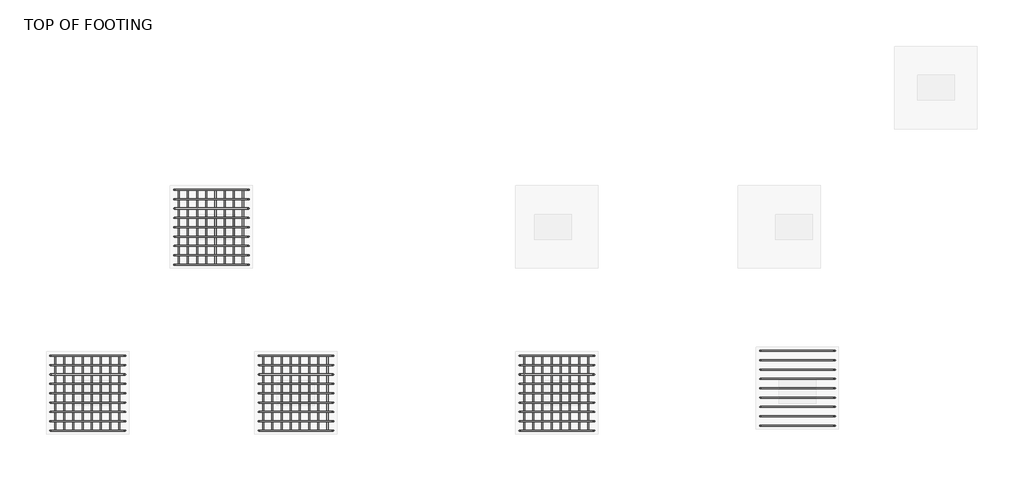
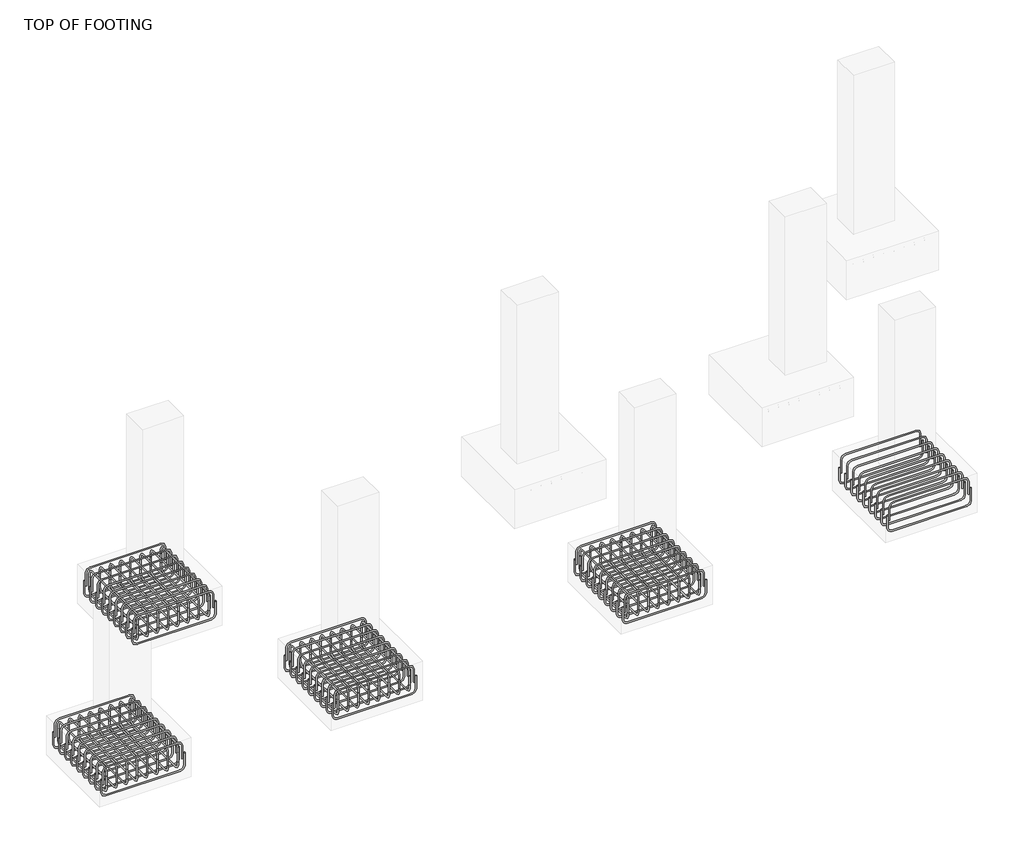
# One storey, part 9 of 20: 18 reinforcing bars.
"""IFC4 building model written with IfcOpenShell, lengths in millimetres."""

from ifc_helpers import new_model, si_unit, point, frame, origin, place, context, project, spatial, polyline, circle_curve, trimmed, segment, composite_curve, source, transform, mapped, element, save
from ifc_brep_helpers import swept_disk

model = new_model("IFC4")

# Units and contexts
model_context = context("Model", 3, world=origin())
ifc_project = project(units=[si_unit("LENGTHUNIT", "METRE", prefix="MILLI")], contexts=[model_context])

# Site, building, storey
site = spatial("IfcSite", under=ifc_project)
building = spatial("IfcBuilding", under=site)
storey = spatial("IfcBuildingStorey", under=building, Name="TOP OF FOOTING", Elevation=-1828.8)

# Reinforcing bars
placement = place(None, origin())
reinforcing_bar_shape = source(origin(), model_context, "Body", "SolidModel", [
    swept_disk(composite_curve([segment(polyline([(6136.1748054, -2535.8035766, -2006.6587682), (6136.1748054, -2535.8035766, -2153.9587682)]), True, "CONTINUOUS"), segment(trimmed(circle_curve(frame((6089.8248054, -2535.8035766, -2153.9587682), z_axis=(0.0, 1.0, 0.0), x_axis=(46.350000000000364, 0.0, 0.0)), 46.35), [point((6136.1748054, -2535.8035766, -2153.9587682))], [point((6089.8248054, -2535.8035766, -2200.3087682))], True, "CARTESIAN"), True, "CONTINUOUS"), segment(polyline([(6089.8248054, -2535.8035766, -2200.3087682), (5275.2248054, -2535.8035766, -2200.3087682)]), True, "CONTINUOUS"), segment(trimmed(circle_curve(frame((5275.2248054, -2535.8035766, -2153.9587682), z_axis=(0.0, 1.0, 0.0), x_axis=(0.0, 0.0, -46.34999999999991)), 46.35), [point((5275.2248054, -2535.8035766, -2200.3087682))], [point((5228.8748054, -2535.8035766, -2153.9587682))], True, "CARTESIAN"), True, "CONTINUOUS"), segment(polyline([(5228.8748054, -2535.8035766, -2153.9587682), (5228.8748054, -2535.8035766, -2006.6587682)]), True, "CONTINUOUS")], self_intersect=False), 6.35),
])
element("IfcReinforcingBar", 1, at=placement, inside=storey, context=model_context, shape_type="MappedRepresentation", body=[
    mapped(reinforcing_bar_shape, transform((0.0, 0.0, 0.0), x_axis=(1.0, 0.0, 0.0), y_axis=(0.0, 1.0, 0.0), z_axis=(0.0, 0.0, 1.0))),
    mapped(reinforcing_bar_shape, transform((0.0, -113.4125, 0.0), x_axis=(1.0, 0.0, 0.0), y_axis=(0.0, 1.0, 0.0), z_axis=(0.0, 0.0, 1.0))),
    mapped(reinforcing_bar_shape, transform((0.0, -226.825, 0.0), x_axis=(1.0, 0.0, 0.0), y_axis=(0.0, 1.0, 0.0), z_axis=(0.0, 0.0, 1.0))),
    mapped(reinforcing_bar_shape, transform((0.0, -340.2375, 0.0), x_axis=(1.0, 0.0, 0.0), y_axis=(0.0, 1.0, 0.0), z_axis=(0.0, 0.0, 1.0))),
    mapped(reinforcing_bar_shape, transform((0.0, -453.65, 0.0), x_axis=(1.0, 0.0, 0.0), y_axis=(0.0, 1.0, 0.0), z_axis=(0.0, 0.0, 1.0))),
    mapped(reinforcing_bar_shape, transform((0.0, -567.0625, 0.0), x_axis=(1.0, 0.0, 0.0), y_axis=(0.0, 1.0, 0.0), z_axis=(0.0, 0.0, 1.0))),
    mapped(reinforcing_bar_shape, transform((0.0, -680.475, 0.0), x_axis=(1.0, 0.0, 0.0), y_axis=(0.0, 1.0, 0.0), z_axis=(0.0, 0.0, 1.0))),
    mapped(reinforcing_bar_shape, transform((0.0, -793.8875, 0.0), x_axis=(1.0, 0.0, 0.0), y_axis=(0.0, 1.0, 0.0), z_axis=(0.0, 0.0, 1.0))),
    mapped(reinforcing_bar_shape, transform((0.0, -907.3, 0.0), x_axis=(1.0, 0.0, 0.0), y_axis=(0.0, 1.0, 0.0), z_axis=(0.0, 0.0, 1.0))),
])
reinforcing_bar_2_shape = source(origin(), model_context, "Body", "SolidModel", [
    swept_disk(composite_curve([segment(polyline([(5248.3489167, -2535.8035766, -2068.8), (5248.3489167, -2535.8035766, -1921.5)]), True, "CONTINUOUS"), segment(trimmed(circle_curve(frame((5294.6989167, -2535.8035766, -1921.5), z_axis=(0.0, 1.0, 0.0), x_axis=(-46.350000000000364, 0.0, 0.0)), 46.35), [point((5248.3489167, -2535.8035766, -1921.5))], [point((5294.6989167, -2535.8035766, -1875.15))], True, "CARTESIAN"), True, "CONTINUOUS"), segment(polyline([(5294.6989167, -2535.8035766, -1875.15), (6064.1623164, -2535.8035766, -1875.15)]), True, "CONTINUOUS"), segment(trimmed(circle_curve(frame((6064.1623164, -2535.8035766, -1921.5), z_axis=(0.0, 1.0, 0.0), x_axis=(0.0, 0.0, 46.34999999999991)), 46.35), [point((6064.1623164, -2535.8035766, -1875.15))], [point((6110.5123164, -2535.8035766, -1921.5))], True, "CARTESIAN"), True, "CONTINUOUS"), segment(polyline([(6110.5123164, -2535.8035766, -1921.5), (6110.5123164, -2535.8035766, -2068.8)]), True, "CONTINUOUS")], self_intersect=False), 6.35),
])
element("IfcReinforcingBar", 2, at=placement, inside=storey, context=model_context, shape_type="MappedRepresentation", body=[
    mapped(reinforcing_bar_2_shape, transform((0.0, 0.0, 0.0), x_axis=(1.0, 0.0, 0.0), y_axis=(0.0, 1.0, 0.0), z_axis=(0.0, 0.0, 1.0))),
    mapped(reinforcing_bar_2_shape, transform((0.0, -113.4125, 0.0), x_axis=(1.0, 0.0, 0.0), y_axis=(0.0, 1.0, 0.0), z_axis=(0.0, 0.0, 1.0))),
    mapped(reinforcing_bar_2_shape, transform((0.0, -226.825, 0.0), x_axis=(1.0, 0.0, 0.0), y_axis=(0.0, 1.0, 0.0), z_axis=(0.0, 0.0, 1.0))),
    mapped(reinforcing_bar_2_shape, transform((0.0, -340.2375, 0.0), x_axis=(1.0, 0.0, 0.0), y_axis=(0.0, 1.0, 0.0), z_axis=(0.0, 0.0, 1.0))),
    mapped(reinforcing_bar_2_shape, transform((0.0, -453.65, 0.0), x_axis=(1.0, 0.0, 0.0), y_axis=(0.0, 1.0, 0.0), z_axis=(0.0, 0.0, 1.0))),
    mapped(reinforcing_bar_2_shape, transform((0.0, -567.0625, 0.0), x_axis=(1.0, 0.0, 0.0), y_axis=(0.0, 1.0, 0.0), z_axis=(0.0, 0.0, 1.0))),
    mapped(reinforcing_bar_2_shape, transform((0.0, -680.475, 0.0), x_axis=(1.0, 0.0, 0.0), y_axis=(0.0, 1.0, 0.0), z_axis=(0.0, 0.0, 1.0))),
    mapped(reinforcing_bar_2_shape, transform((0.0, -793.8875, 0.0), x_axis=(1.0, 0.0, 0.0), y_axis=(0.0, 1.0, 0.0), z_axis=(0.0, 0.0, 1.0))),
    mapped(reinforcing_bar_2_shape, transform((0.0, -907.3, 0.0), x_axis=(1.0, 0.0, 0.0), y_axis=(0.0, 1.0, 0.0), z_axis=(0.0, 0.0, 1.0))),
])
reinforcing_bar_3_shape = source(origin(), model_context, "Body", "SolidModel", [
    swept_disk(composite_curve([segment(polyline([(6064.677844, -2535.8035766, -2086.1951968), (6064.677844, -2535.8035766, -1938.8951968)]), True, "CONTINUOUS"), segment(trimmed(circle_curve(frame((6064.677844, -2582.1535766, -1938.8951968), z_axis=(1.0, 0.0, 0.0), x_axis=(0.0, 46.350000000000364, 0.0)), 46.35), [point((6064.677844, -2535.8035766, -1938.8951968))], [point((6064.677844, -2582.1535766, -1892.5451968))], True, "CARTESIAN"), True, "CONTINUOUS"), segment(polyline([(6064.677844, -2582.1535766, -1892.5451968), (6064.677844, -3396.7535766, -1892.5451968)]), True, "CONTINUOUS"), segment(trimmed(circle_curve(frame((6064.677844, -3396.7535766, -1938.8951968), z_axis=(1.0, 0.0, 0.0), x_axis=(0.0, 0.0, 46.34999999999991)), 46.35), [point((6064.677844, -3396.7535766, -1892.5451968))], [point((6064.677844, -3443.1035766, -1938.8951968))], True, "CARTESIAN"), True, "CONTINUOUS"), segment(polyline([(6064.677844, -3443.1035766, -1938.8951968), (6064.677844, -3443.1035766, -2086.1951968)]), True, "CONTINUOUS")], self_intersect=False), 6.35),
])
element("IfcReinforcingBar", 3, at=placement, inside=storey, context=model_context, shape_type="MappedRepresentation", body=[
    mapped(reinforcing_bar_3_shape, transform((0.0, 0.0, 0.0), x_axis=(1.0, 0.0, 0.0), y_axis=(0.0, 1.0, 0.0), z_axis=(0.0, 0.0, 1.0))),
    mapped(reinforcing_bar_3_shape, transform((-111.2862402, 0.0, 0.0), x_axis=(1.0, 0.0, 0.0), y_axis=(0.0, 1.0, 0.0), z_axis=(0.0, 0.0, 1.0))),
    mapped(reinforcing_bar_3_shape, transform((-222.5724804, 0.0, 0.0), x_axis=(1.0, 0.0, 0.0), y_axis=(0.0, 1.0, 0.0), z_axis=(0.0, 0.0, 1.0))),
    mapped(reinforcing_bar_3_shape, transform((-333.8587205, 0.0, 0.0), x_axis=(1.0, 0.0, 0.0), y_axis=(0.0, 1.0, 0.0), z_axis=(0.0, 0.0, 1.0))),
    mapped(reinforcing_bar_3_shape, transform((-445.1449607, 0.0, 0.0), x_axis=(1.0, 0.0, 0.0), y_axis=(0.0, 1.0, 0.0), z_axis=(0.0, 0.0, 1.0))),
    mapped(reinforcing_bar_3_shape, transform((-556.4312009, 0.0, 0.0), x_axis=(1.0, 0.0, 0.0), y_axis=(0.0, 1.0, 0.0), z_axis=(0.0, 0.0, 1.0))),
    mapped(reinforcing_bar_3_shape, transform((-667.7174411, 0.0, 0.0), x_axis=(1.0, 0.0, 0.0), y_axis=(0.0, 1.0, 0.0), z_axis=(0.0, 0.0, 1.0))),
    mapped(reinforcing_bar_3_shape, transform((-779.0036813, 0.0, 0.0), x_axis=(1.0, 0.0, 0.0), y_axis=(0.0, 1.0, 0.0), z_axis=(0.0, 0.0, 1.0))),
])
reinforcing_bar_4_shape = source(origin(), model_context, "Body", "SolidModel", [
    swept_disk(composite_curve([segment(polyline([(5285.6741627, -2535.8035766, -1979.1645013), (5285.6741627, -2535.8035766, -2126.4645013)]), True, "CONTINUOUS"), segment(trimmed(circle_curve(frame((5285.6741627, -2582.1535766, -2126.4645013), z_axis=(-1.0, 0.0, 0.0), x_axis=(0.0, 46.350000000000364, 0.0)), 46.35), [point((5285.6741627, -2535.8035766, -2126.4645013))], [point((5285.6741627, -2582.1535766, -2172.8145013))], True, "CARTESIAN"), True, "CONTINUOUS"), segment(polyline([(5285.6741627, -2582.1535766, -2172.8145013), (5285.6741627, -3396.7535766, -2172.8145013)]), True, "CONTINUOUS"), segment(trimmed(circle_curve(frame((5285.6741627, -3396.7535766, -2126.4645013), z_axis=(-1.0, 0.0, 0.0), x_axis=(0.0, 0.0, -46.34999999999991)), 46.35), [point((5285.6741627, -3396.7535766, -2172.8145013))], [point((5285.6741627, -3443.1035766, -2126.4645013))], True, "CARTESIAN"), True, "CONTINUOUS"), segment(polyline([(5285.6741627, -3443.1035766, -2126.4645013), (5285.6741627, -3443.1035766, -1979.1645013)]), True, "CONTINUOUS")], self_intersect=False), 6.35),
])
element("IfcReinforcingBar", 4, at=placement, inside=storey, context=model_context, shape_type="MappedRepresentation", body=[
    mapped(reinforcing_bar_4_shape, transform((0.0, 0.0, 0.0), x_axis=(1.0, 0.0, 0.0), y_axis=(0.0, 1.0, 0.0), z_axis=(0.0, 0.0, 1.0))),
    mapped(reinforcing_bar_4_shape, transform((111.2862402, 0.0, 0.0), x_axis=(1.0, 0.0, 0.0), y_axis=(0.0, 1.0, 0.0), z_axis=(0.0, 0.0, 1.0))),
    mapped(reinforcing_bar_4_shape, transform((222.5724804, 0.0, 0.0), x_axis=(1.0, 0.0, 0.0), y_axis=(0.0, 1.0, 0.0), z_axis=(0.0, 0.0, 1.0))),
    mapped(reinforcing_bar_4_shape, transform((333.8587205, 0.0, 0.0), x_axis=(1.0, 0.0, 0.0), y_axis=(0.0, 1.0, 0.0), z_axis=(0.0, 0.0, 1.0))),
    mapped(reinforcing_bar_4_shape, transform((445.1449607, 0.0, 0.0), x_axis=(1.0, 0.0, 0.0), y_axis=(0.0, 1.0, 0.0), z_axis=(0.0, 0.0, 1.0))),
    mapped(reinforcing_bar_4_shape, transform((556.4312009, 0.0, 0.0), x_axis=(1.0, 0.0, 0.0), y_axis=(0.0, 1.0, 0.0), z_axis=(0.0, 0.0, 1.0))),
    mapped(reinforcing_bar_4_shape, transform((667.7174411, 0.0, 0.0), x_axis=(1.0, 0.0, 0.0), y_axis=(0.0, 1.0, 0.0), z_axis=(0.0, 0.0, 1.0))),
    mapped(reinforcing_bar_4_shape, transform((779.0036813, 0.0, 0.0), x_axis=(1.0, 0.0, 0.0), y_axis=(0.0, 1.0, 0.0), z_axis=(0.0, 0.0, 1.0))),
])
reinforcing_bar_5_shape = source(origin(), model_context, "Body", "SolidModel", [
    swept_disk(composite_curve([segment(polyline([(7160.5179014, -4547.9729916, -2006.6587682), (7160.5179014, -4547.9729916, -2153.9587682)]), True, "CONTINUOUS"), segment(trimmed(circle_curve(frame((7114.1679014, -4547.9729916, -2153.9587682), z_axis=(0.0, 1.0, 0.0), x_axis=(46.349999999999454, 0.0, 0.0)), 46.35), [point((7160.5179014, -4547.9729916, -2153.9587682))], [point((7114.1679014, -4547.9729916, -2200.3087682))], True, "CARTESIAN"), True, "CONTINUOUS"), segment(polyline([(7114.1679014, -4547.9729916, -2200.3087682), (6299.5679014, -4547.9729916, -2200.3087682)]), True, "CONTINUOUS"), segment(trimmed(circle_curve(frame((6299.5679014, -4547.9729916, -2153.9587682), z_axis=(0.0, 1.0, 0.0), x_axis=(0.0, 0.0, -46.34999999999991)), 46.35), [point((6299.5679014, -4547.9729916, -2200.3087682))], [point((6253.2179014, -4547.9729916, -2153.9587682))], True, "CARTESIAN"), True, "CONTINUOUS"), segment(polyline([(6253.2179014, -4547.9729916, -2153.9587682), (6253.2179014, -4547.9729916, -2006.6587682)]), True, "CONTINUOUS")], self_intersect=False), 6.35),
])
element("IfcReinforcingBar", 5, at=placement, inside=storey, context=model_context, shape_type="MappedRepresentation", body=[
    mapped(reinforcing_bar_5_shape, transform((0.0, 0.0, 0.0), x_axis=(1.0, 0.0, 0.0), y_axis=(0.0, 1.0, 0.0), z_axis=(0.0, 0.0, 1.0))),
    mapped(reinforcing_bar_5_shape, transform((0.0, -113.4125, 0.0), x_axis=(1.0, 0.0, 0.0), y_axis=(0.0, 1.0, 0.0), z_axis=(0.0, 0.0, 1.0))),
    mapped(reinforcing_bar_5_shape, transform((0.0, -226.825, 0.0), x_axis=(1.0, 0.0, 0.0), y_axis=(0.0, 1.0, 0.0), z_axis=(0.0, 0.0, 1.0))),
    mapped(reinforcing_bar_5_shape, transform((0.0, -340.2375, 0.0), x_axis=(1.0, 0.0, 0.0), y_axis=(0.0, 1.0, 0.0), z_axis=(0.0, 0.0, 1.0))),
    mapped(reinforcing_bar_5_shape, transform((0.0, -453.65, 0.0), x_axis=(1.0, 0.0, 0.0), y_axis=(0.0, 1.0, 0.0), z_axis=(0.0, 0.0, 1.0))),
    mapped(reinforcing_bar_5_shape, transform((0.0, -567.0625, 0.0), x_axis=(1.0, 0.0, 0.0), y_axis=(0.0, 1.0, 0.0), z_axis=(0.0, 0.0, 1.0))),
    mapped(reinforcing_bar_5_shape, transform((0.0, -680.475, 0.0), x_axis=(1.0, 0.0, 0.0), y_axis=(0.0, 1.0, 0.0), z_axis=(0.0, 0.0, 1.0))),
    mapped(reinforcing_bar_5_shape, transform((0.0, -793.8875, 0.0), x_axis=(1.0, 0.0, 0.0), y_axis=(0.0, 1.0, 0.0), z_axis=(0.0, 0.0, 1.0))),
    mapped(reinforcing_bar_5_shape, transform((0.0, -907.3, 0.0), x_axis=(1.0, 0.0, 0.0), y_axis=(0.0, 1.0, 0.0), z_axis=(0.0, 0.0, 1.0))),
])
reinforcing_bar_6_shape = source(origin(), model_context, "Body", "SolidModel", [
    swept_disk(composite_curve([segment(polyline([(6272.6920127, -4547.9729916, -2068.8), (6272.6920127, -4547.9729916, -1921.5)]), True, "CONTINUOUS"), segment(trimmed(circle_curve(frame((6319.0420127, -4547.9729916, -1921.5), z_axis=(0.0, 1.0, 0.0), x_axis=(-46.349999999999454, 0.0, 0.0)), 46.35), [point((6272.6920127, -4547.9729916, -1921.5))], [point((6319.0420127, -4547.9729916, -1875.15))], True, "CARTESIAN"), True, "CONTINUOUS"), segment(polyline([(6319.0420127, -4547.9729916, -1875.15), (7088.5054124, -4547.9729916, -1875.15)]), True, "CONTINUOUS"), segment(trimmed(circle_curve(frame((7088.5054124, -4547.9729916, -1921.5), z_axis=(0.0, 1.0, 0.0), x_axis=(0.0, 0.0, 46.34999999999991)), 46.35), [point((7088.5054124, -4547.9729916, -1875.15))], [point((7134.8554124, -4547.9729916, -1921.5))], True, "CARTESIAN"), True, "CONTINUOUS"), segment(polyline([(7134.8554124, -4547.9729916, -1921.5), (7134.8554124, -4547.9729916, -2068.8)]), True, "CONTINUOUS")], self_intersect=False), 6.35),
])
element("IfcReinforcingBar", 6, at=placement, inside=storey, context=model_context, shape_type="MappedRepresentation", body=[
    mapped(reinforcing_bar_6_shape, transform((0.0, 0.0, 0.0), x_axis=(1.0, 0.0, 0.0), y_axis=(0.0, 1.0, 0.0), z_axis=(0.0, 0.0, 1.0))),
    mapped(reinforcing_bar_6_shape, transform((0.0, -113.4125, 0.0), x_axis=(1.0, 0.0, 0.0), y_axis=(0.0, 1.0, 0.0), z_axis=(0.0, 0.0, 1.0))),
    mapped(reinforcing_bar_6_shape, transform((0.0, -226.825, 0.0), x_axis=(1.0, 0.0, 0.0), y_axis=(0.0, 1.0, 0.0), z_axis=(0.0, 0.0, 1.0))),
    mapped(reinforcing_bar_6_shape, transform((0.0, -340.2375, 0.0), x_axis=(1.0, 0.0, 0.0), y_axis=(0.0, 1.0, 0.0), z_axis=(0.0, 0.0, 1.0))),
    mapped(reinforcing_bar_6_shape, transform((0.0, -453.65, 0.0), x_axis=(1.0, 0.0, 0.0), y_axis=(0.0, 1.0, 0.0), z_axis=(0.0, 0.0, 1.0))),
    mapped(reinforcing_bar_6_shape, transform((0.0, -567.0625, 0.0), x_axis=(1.0, 0.0, 0.0), y_axis=(0.0, 1.0, 0.0), z_axis=(0.0, 0.0, 1.0))),
    mapped(reinforcing_bar_6_shape, transform((0.0, -680.475, 0.0), x_axis=(1.0, 0.0, 0.0), y_axis=(0.0, 1.0, 0.0), z_axis=(0.0, 0.0, 1.0))),
    mapped(reinforcing_bar_6_shape, transform((0.0, -793.8875, 0.0), x_axis=(1.0, 0.0, 0.0), y_axis=(0.0, 1.0, 0.0), z_axis=(0.0, 0.0, 1.0))),
    mapped(reinforcing_bar_6_shape, transform((0.0, -907.3, 0.0), x_axis=(1.0, 0.0, 0.0), y_axis=(0.0, 1.0, 0.0), z_axis=(0.0, 0.0, 1.0))),
])
reinforcing_bar_7_shape = source(origin(), model_context, "Body", "SolidModel", [
    swept_disk(composite_curve([segment(polyline([(7089.02094, -4547.9729916, -2086.1951968), (7089.02094, -4547.9729916, -1938.8951968)]), True, "CONTINUOUS"), segment(trimmed(circle_curve(frame((7089.02094, -4594.3229916, -1938.8951968), z_axis=(1.0, 0.0, 0.0), x_axis=(0.0, 46.350000000000364, 0.0)), 46.35), [point((7089.02094, -4547.9729916, -1938.8951968))], [point((7089.02094, -4594.3229916, -1892.5451968))], True, "CARTESIAN"), True, "CONTINUOUS"), segment(polyline([(7089.02094, -4594.3229916, -1892.5451968), (7089.02094, -5408.9229916, -1892.5451968)]), True, "CONTINUOUS"), segment(trimmed(circle_curve(frame((7089.02094, -5408.9229916, -1938.8951968), z_axis=(1.0, 0.0, 0.0), x_axis=(0.0, 0.0, 46.34999999999991)), 46.35), [point((7089.02094, -5408.9229916, -1892.5451968))], [point((7089.02094, -5455.2729916, -1938.8951968))], True, "CARTESIAN"), True, "CONTINUOUS"), segment(polyline([(7089.02094, -5455.2729916, -1938.8951968), (7089.02094, -5455.2729916, -2086.1951968)]), True, "CONTINUOUS")], self_intersect=False), 6.35),
])
element("IfcReinforcingBar", 7, at=placement, inside=storey, context=model_context, shape_type="MappedRepresentation", body=[
    mapped(reinforcing_bar_7_shape, transform((0.0, 0.0, 0.0), x_axis=(1.0, 0.0, 0.0), y_axis=(0.0, 1.0, 0.0), z_axis=(0.0, 0.0, 1.0))),
    mapped(reinforcing_bar_7_shape, transform((-111.2862402, 0.0, 0.0), x_axis=(1.0, 0.0, 0.0), y_axis=(0.0, 1.0, 0.0), z_axis=(0.0, 0.0, 1.0))),
    mapped(reinforcing_bar_7_shape, transform((-222.5724804, 0.0, 0.0), x_axis=(1.0, 0.0, 0.0), y_axis=(0.0, 1.0, 0.0), z_axis=(0.0, 0.0, 1.0))),
    mapped(reinforcing_bar_7_shape, transform((-333.8587205, 0.0, 0.0), x_axis=(1.0, 0.0, 0.0), y_axis=(0.0, 1.0, 0.0), z_axis=(0.0, 0.0, 1.0))),
    mapped(reinforcing_bar_7_shape, transform((-445.1449607, 0.0, 0.0), x_axis=(1.0, 0.0, 0.0), y_axis=(0.0, 1.0, 0.0), z_axis=(0.0, 0.0, 1.0))),
    mapped(reinforcing_bar_7_shape, transform((-556.4312009, 0.0, 0.0), x_axis=(1.0, 0.0, 0.0), y_axis=(0.0, 1.0, 0.0), z_axis=(0.0, 0.0, 1.0))),
    mapped(reinforcing_bar_7_shape, transform((-667.7174411, 0.0, 0.0), x_axis=(1.0, 0.0, 0.0), y_axis=(0.0, 1.0, 0.0), z_axis=(0.0, 0.0, 1.0))),
    mapped(reinforcing_bar_7_shape, transform((-779.0036813, 0.0, 0.0), x_axis=(1.0, 0.0, 0.0), y_axis=(0.0, 1.0, 0.0), z_axis=(0.0, 0.0, 1.0))),
])
reinforcing_bar_8_shape = source(origin(), model_context, "Body", "SolidModel", [
    swept_disk(composite_curve([segment(polyline([(6310.0172587, -4547.9729916, -1979.1645013), (6310.0172587, -4547.9729916, -2126.4645013)]), True, "CONTINUOUS"), segment(trimmed(circle_curve(frame((6310.0172587, -4594.3229916, -2126.4645013), z_axis=(-1.0, 0.0, 0.0), x_axis=(0.0, 46.350000000000364, 0.0)), 46.35), [point((6310.0172587, -4547.9729916, -2126.4645013))], [point((6310.0172587, -4594.3229916, -2172.8145013))], True, "CARTESIAN"), True, "CONTINUOUS"), segment(polyline([(6310.0172587, -4594.3229916, -2172.8145013), (6310.0172587, -5408.9229916, -2172.8145013)]), True, "CONTINUOUS"), segment(trimmed(circle_curve(frame((6310.0172587, -5408.9229916, -2126.4645013), z_axis=(-1.0, 0.0, 0.0), x_axis=(0.0, 0.0, -46.34999999999991)), 46.35), [point((6310.0172587, -5408.9229916, -2172.8145013))], [point((6310.0172587, -5455.2729916, -2126.4645013))], True, "CARTESIAN"), True, "CONTINUOUS"), segment(polyline([(6310.0172587, -5455.2729916, -2126.4645013), (6310.0172587, -5455.2729916, -1979.1645013)]), True, "CONTINUOUS")], self_intersect=False), 6.35),
])
element("IfcReinforcingBar", 8, at=placement, inside=storey, context=model_context, shape_type="MappedRepresentation", body=[
    mapped(reinforcing_bar_8_shape, transform((0.0, 0.0, 0.0), x_axis=(1.0, 0.0, 0.0), y_axis=(0.0, 1.0, 0.0), z_axis=(0.0, 0.0, 1.0))),
    mapped(reinforcing_bar_8_shape, transform((111.2862402, 0.0, 0.0), x_axis=(1.0, 0.0, 0.0), y_axis=(0.0, 1.0, 0.0), z_axis=(0.0, 0.0, 1.0))),
    mapped(reinforcing_bar_8_shape, transform((222.5724804, 0.0, 0.0), x_axis=(1.0, 0.0, 0.0), y_axis=(0.0, 1.0, 0.0), z_axis=(0.0, 0.0, 1.0))),
    mapped(reinforcing_bar_8_shape, transform((333.8587205, 0.0, 0.0), x_axis=(1.0, 0.0, 0.0), y_axis=(0.0, 1.0, 0.0), z_axis=(0.0, 0.0, 1.0))),
    mapped(reinforcing_bar_8_shape, transform((445.1449607, 0.0, 0.0), x_axis=(1.0, 0.0, 0.0), y_axis=(0.0, 1.0, 0.0), z_axis=(0.0, 0.0, 1.0))),
    mapped(reinforcing_bar_8_shape, transform((556.4312009, 0.0, 0.0), x_axis=(1.0, 0.0, 0.0), y_axis=(0.0, 1.0, 0.0), z_axis=(0.0, 0.0, 1.0))),
    mapped(reinforcing_bar_8_shape, transform((667.7174411, 0.0, 0.0), x_axis=(1.0, 0.0, 0.0), y_axis=(0.0, 1.0, 0.0), z_axis=(0.0, 0.0, 1.0))),
    mapped(reinforcing_bar_8_shape, transform((779.0036813, 0.0, 0.0), x_axis=(1.0, 0.0, 0.0), y_axis=(0.0, 1.0, 0.0), z_axis=(0.0, 0.0, 1.0))),
])
reinforcing_bar_9_shape = source(origin(), model_context, "Body", "SolidModel", [
    swept_disk(composite_curve([segment(polyline([(10322.7663908, -4547.9729916, -2006.6587682), (10322.7663908, -4547.9729916, -2153.9587682)]), True, "CONTINUOUS"), segment(trimmed(circle_curve(frame((10276.4163908, -4547.9729916, -2153.9587682), z_axis=(0.0, 1.0, 0.0), x_axis=(46.350000000000364, 0.0, 0.0)), 46.35), [point((10322.7663908, -4547.9729916, -2153.9587682))], [point((10276.4163908, -4547.9729916, -2200.3087682))], True, "CARTESIAN"), True, "CONTINUOUS"), segment(polyline([(10276.4163908, -4547.9729916, -2200.3087682), (9461.8163908, -4547.9729916, -2200.3087682)]), True, "CONTINUOUS"), segment(trimmed(circle_curve(frame((9461.8163908, -4547.9729916, -2153.9587682), z_axis=(0.0, 1.0, 0.0), x_axis=(0.0, 0.0, -46.34999999999991)), 46.35), [point((9461.8163908, -4547.9729916, -2200.3087682))], [point((9415.4663908, -4547.9729916, -2153.9587682))], True, "CARTESIAN"), True, "CONTINUOUS"), segment(polyline([(9415.4663908, -4547.9729916, -2153.9587682), (9415.4663908, -4547.9729916, -2006.6587682)]), True, "CONTINUOUS")], self_intersect=False), 6.35),
])
element("IfcReinforcingBar", 9, at=placement, inside=storey, context=model_context, shape_type="MappedRepresentation", body=[
    mapped(reinforcing_bar_9_shape, transform((0.0, 0.0, 0.0), x_axis=(1.0, 0.0, 0.0), y_axis=(0.0, 1.0, 0.0), z_axis=(0.0, 0.0, 1.0))),
    mapped(reinforcing_bar_9_shape, transform((0.0, -113.4125, 0.0), x_axis=(1.0, 0.0, 0.0), y_axis=(0.0, 1.0, 0.0), z_axis=(0.0, 0.0, 1.0))),
    mapped(reinforcing_bar_9_shape, transform((0.0, -226.825, 0.0), x_axis=(1.0, 0.0, 0.0), y_axis=(0.0, 1.0, 0.0), z_axis=(0.0, 0.0, 1.0))),
    mapped(reinforcing_bar_9_shape, transform((0.0, -340.2375, 0.0), x_axis=(1.0, 0.0, 0.0), y_axis=(0.0, 1.0, 0.0), z_axis=(0.0, 0.0, 1.0))),
    mapped(reinforcing_bar_9_shape, transform((0.0, -453.65, 0.0), x_axis=(1.0, 0.0, 0.0), y_axis=(0.0, 1.0, 0.0), z_axis=(0.0, 0.0, 1.0))),
    mapped(reinforcing_bar_9_shape, transform((0.0, -567.0625, 0.0), x_axis=(1.0, 0.0, 0.0), y_axis=(0.0, 1.0, 0.0), z_axis=(0.0, 0.0, 1.0))),
    mapped(reinforcing_bar_9_shape, transform((0.0, -680.475, 0.0), x_axis=(1.0, 0.0, 0.0), y_axis=(0.0, 1.0, 0.0), z_axis=(0.0, 0.0, 1.0))),
    mapped(reinforcing_bar_9_shape, transform((0.0, -793.8875, 0.0), x_axis=(1.0, 0.0, 0.0), y_axis=(0.0, 1.0, 0.0), z_axis=(0.0, 0.0, 1.0))),
    mapped(reinforcing_bar_9_shape, transform((0.0, -907.3, 0.0), x_axis=(1.0, 0.0, 0.0), y_axis=(0.0, 1.0, 0.0), z_axis=(0.0, 0.0, 1.0))),
])
reinforcing_bar_10_shape = source(origin(), model_context, "Body", "SolidModel", [
    swept_disk(composite_curve([segment(polyline([(9434.9405021, -4547.9729916, -2068.8), (9434.9405021, -4547.9729916, -1921.5)]), True, "CONTINUOUS"), segment(trimmed(circle_curve(frame((9481.2905021, -4547.9729916, -1921.5), z_axis=(0.0, 1.0, 0.0), x_axis=(-46.350000000000364, 0.0, 0.0)), 46.35), [point((9434.9405021, -4547.9729916, -1921.5))], [point((9481.2905021, -4547.9729916, -1875.15))], True, "CARTESIAN"), True, "CONTINUOUS"), segment(polyline([(9481.2905021, -4547.9729916, -1875.15), (10250.7539017, -4547.9729916, -1875.15)]), True, "CONTINUOUS"), segment(trimmed(circle_curve(frame((10250.7539017, -4547.9729916, -1921.5), z_axis=(0.0, 1.0, 0.0), x_axis=(0.0, 0.0, 46.34999999999991)), 46.35), [point((10250.7539017, -4547.9729916, -1875.15))], [point((10297.1039017, -4547.9729916, -1921.5))], True, "CARTESIAN"), True, "CONTINUOUS"), segment(polyline([(10297.1039017, -4547.9729916, -1921.5), (10297.1039017, -4547.9729916, -2068.8)]), True, "CONTINUOUS")], self_intersect=False), 6.35),
])
element("IfcReinforcingBar", 10, at=placement, inside=storey, context=model_context, shape_type="MappedRepresentation", body=[
    mapped(reinforcing_bar_10_shape, transform((0.0, 0.0, 0.0), x_axis=(1.0, 0.0, 0.0), y_axis=(0.0, 1.0, 0.0), z_axis=(0.0, 0.0, 1.0))),
    mapped(reinforcing_bar_10_shape, transform((0.0, -113.4125, 0.0), x_axis=(1.0, 0.0, 0.0), y_axis=(0.0, 1.0, 0.0), z_axis=(0.0, 0.0, 1.0))),
    mapped(reinforcing_bar_10_shape, transform((0.0, -226.825, 0.0), x_axis=(1.0, 0.0, 0.0), y_axis=(0.0, 1.0, 0.0), z_axis=(0.0, 0.0, 1.0))),
    mapped(reinforcing_bar_10_shape, transform((0.0, -340.2375, 0.0), x_axis=(1.0, 0.0, 0.0), y_axis=(0.0, 1.0, 0.0), z_axis=(0.0, 0.0, 1.0))),
    mapped(reinforcing_bar_10_shape, transform((0.0, -453.65, 0.0), x_axis=(1.0, 0.0, 0.0), y_axis=(0.0, 1.0, 0.0), z_axis=(0.0, 0.0, 1.0))),
    mapped(reinforcing_bar_10_shape, transform((0.0, -567.0625, 0.0), x_axis=(1.0, 0.0, 0.0), y_axis=(0.0, 1.0, 0.0), z_axis=(0.0, 0.0, 1.0))),
    mapped(reinforcing_bar_10_shape, transform((0.0, -680.475, 0.0), x_axis=(1.0, 0.0, 0.0), y_axis=(0.0, 1.0, 0.0), z_axis=(0.0, 0.0, 1.0))),
    mapped(reinforcing_bar_10_shape, transform((0.0, -793.8875, 0.0), x_axis=(1.0, 0.0, 0.0), y_axis=(0.0, 1.0, 0.0), z_axis=(0.0, 0.0, 1.0))),
    mapped(reinforcing_bar_10_shape, transform((0.0, -907.3, 0.0), x_axis=(1.0, 0.0, 0.0), y_axis=(0.0, 1.0, 0.0), z_axis=(0.0, 0.0, 1.0))),
])
reinforcing_bar_11_shape = source(origin(), model_context, "Body", "SolidModel", [
    swept_disk(composite_curve([segment(polyline([(10251.2694294, -4547.9729916, -2086.1951968), (10251.2694294, -4547.9729916, -1938.8951968)]), True, "CONTINUOUS"), segment(trimmed(circle_curve(frame((10251.2694294, -4594.3229916, -1938.8951968), z_axis=(1.0, 0.0, 0.0), x_axis=(0.0, 46.350000000000364, 0.0)), 46.35), [point((10251.2694294, -4547.9729916, -1938.8951968))], [point((10251.2694294, -4594.3229916, -1892.5451968))], True, "CARTESIAN"), True, "CONTINUOUS"), segment(polyline([(10251.2694294, -4594.3229916, -1892.5451968), (10251.2694294, -5408.9229916, -1892.5451968)]), True, "CONTINUOUS"), segment(trimmed(circle_curve(frame((10251.2694294, -5408.9229916, -1938.8951968), z_axis=(1.0, 0.0, 0.0), x_axis=(0.0, 0.0, 46.34999999999991)), 46.35), [point((10251.2694294, -5408.9229916, -1892.5451968))], [point((10251.2694294, -5455.2729916, -1938.8951968))], True, "CARTESIAN"), True, "CONTINUOUS"), segment(polyline([(10251.2694294, -5455.2729916, -1938.8951968), (10251.2694294, -5455.2729916, -2086.1951968)]), True, "CONTINUOUS")], self_intersect=False), 6.35),
])
element("IfcReinforcingBar", 11, at=placement, inside=storey, context=model_context, shape_type="MappedRepresentation", body=[
    mapped(reinforcing_bar_11_shape, transform((0.0, 0.0, 0.0), x_axis=(1.0, 0.0, 0.0), y_axis=(0.0, 1.0, 0.0), z_axis=(0.0, 0.0, 1.0))),
    mapped(reinforcing_bar_11_shape, transform((-111.2862402, 0.0, 0.0), x_axis=(1.0, 0.0, 0.0), y_axis=(0.0, 1.0, 0.0), z_axis=(0.0, 0.0, 1.0))),
    mapped(reinforcing_bar_11_shape, transform((-222.5724804, 0.0, 0.0), x_axis=(1.0, 0.0, 0.0), y_axis=(0.0, 1.0, 0.0), z_axis=(0.0, 0.0, 1.0))),
    mapped(reinforcing_bar_11_shape, transform((-333.8587205, 0.0, 0.0), x_axis=(1.0, 0.0, 0.0), y_axis=(0.0, 1.0, 0.0), z_axis=(0.0, 0.0, 1.0))),
    mapped(reinforcing_bar_11_shape, transform((-445.1449607, 0.0, 0.0), x_axis=(1.0, 0.0, 0.0), y_axis=(0.0, 1.0, 0.0), z_axis=(0.0, 0.0, 1.0))),
    mapped(reinforcing_bar_11_shape, transform((-556.4312009, 0.0, 0.0), x_axis=(1.0, 0.0, 0.0), y_axis=(0.0, 1.0, 0.0), z_axis=(0.0, 0.0, 1.0))),
    mapped(reinforcing_bar_11_shape, transform((-667.7174411, 0.0, 0.0), x_axis=(1.0, 0.0, 0.0), y_axis=(0.0, 1.0, 0.0), z_axis=(0.0, 0.0, 1.0))),
    mapped(reinforcing_bar_11_shape, transform((-779.0036813, 0.0, 0.0), x_axis=(1.0, 0.0, 0.0), y_axis=(0.0, 1.0, 0.0), z_axis=(0.0, 0.0, 1.0))),
])
reinforcing_bar_12_shape = source(origin(), model_context, "Body", "SolidModel", [
    swept_disk(composite_curve([segment(polyline([(9472.2657481, -4547.9729916, -1979.1645013), (9472.2657481, -4547.9729916, -2126.4645013)]), True, "CONTINUOUS"), segment(trimmed(circle_curve(frame((9472.2657481, -4594.3229916, -2126.4645013), z_axis=(-1.0, 0.0, 0.0), x_axis=(0.0, 46.350000000000364, 0.0)), 46.35), [point((9472.2657481, -4547.9729916, -2126.4645013))], [point((9472.2657481, -4594.3229916, -2172.8145013))], True, "CARTESIAN"), True, "CONTINUOUS"), segment(polyline([(9472.2657481, -4594.3229916, -2172.8145013), (9472.2657481, -5408.9229916, -2172.8145013)]), True, "CONTINUOUS"), segment(trimmed(circle_curve(frame((9472.2657481, -5408.9229916, -2126.4645013), z_axis=(-1.0, 0.0, 0.0), x_axis=(0.0, 0.0, -46.34999999999991)), 46.35), [point((9472.2657481, -5408.9229916, -2172.8145013))], [point((9472.2657481, -5455.2729916, -2126.4645013))], True, "CARTESIAN"), True, "CONTINUOUS"), segment(polyline([(9472.2657481, -5455.2729916, -2126.4645013), (9472.2657481, -5455.2729916, -1979.1645013)]), True, "CONTINUOUS")], self_intersect=False), 6.35),
])
element("IfcReinforcingBar", 12, at=placement, inside=storey, context=model_context, shape_type="MappedRepresentation", body=[
    mapped(reinforcing_bar_12_shape, transform((0.0, 0.0, 0.0), x_axis=(1.0, 0.0, 0.0), y_axis=(0.0, 1.0, 0.0), z_axis=(0.0, 0.0, 1.0))),
    mapped(reinforcing_bar_12_shape, transform((111.2862402, 0.0, 0.0), x_axis=(1.0, 0.0, 0.0), y_axis=(0.0, 1.0, 0.0), z_axis=(0.0, 0.0, 1.0))),
    mapped(reinforcing_bar_12_shape, transform((222.5724804, 0.0, 0.0), x_axis=(1.0, 0.0, 0.0), y_axis=(0.0, 1.0, 0.0), z_axis=(0.0, 0.0, 1.0))),
    mapped(reinforcing_bar_12_shape, transform((333.8587205, 0.0, 0.0), x_axis=(1.0, 0.0, 0.0), y_axis=(0.0, 1.0, 0.0), z_axis=(0.0, 0.0, 1.0))),
    mapped(reinforcing_bar_12_shape, transform((445.1449607, 0.0, 0.0), x_axis=(1.0, 0.0, 0.0), y_axis=(0.0, 1.0, 0.0), z_axis=(0.0, 0.0, 1.0))),
    mapped(reinforcing_bar_12_shape, transform((556.4312009, 0.0, 0.0), x_axis=(1.0, 0.0, 0.0), y_axis=(0.0, 1.0, 0.0), z_axis=(0.0, 0.0, 1.0))),
    mapped(reinforcing_bar_12_shape, transform((667.7174411, 0.0, 0.0), x_axis=(1.0, 0.0, 0.0), y_axis=(0.0, 1.0, 0.0), z_axis=(0.0, 0.0, 1.0))),
    mapped(reinforcing_bar_12_shape, transform((779.0036813, 0.0, 0.0), x_axis=(1.0, 0.0, 0.0), y_axis=(0.0, 1.0, 0.0), z_axis=(0.0, 0.0, 1.0))),
])
reinforcing_bar_13_shape = source(origin(), model_context, "Body", "SolidModel", [
    swept_disk(composite_curve([segment(polyline([(13242.7663908, -4487.9729916, -2006.6587682), (13242.7663908, -4487.9729916, -2153.9587682)]), True, "CONTINUOUS"), segment(trimmed(circle_curve(frame((13196.4163908, -4487.9729916, -2153.9587682), z_axis=(0.0, 1.0, 0.0), x_axis=(46.350000000000364, 0.0, 0.0)), 46.35), [point((13242.7663908, -4487.9729916, -2153.9587682))], [point((13196.4163908, -4487.9729916, -2200.3087682))], True, "CARTESIAN"), True, "CONTINUOUS"), segment(polyline([(13196.4163908, -4487.9729916, -2200.3087682), (12381.8163908, -4487.9729916, -2200.3087682)]), True, "CONTINUOUS"), segment(trimmed(circle_curve(frame((12381.8163908, -4487.9729916, -2153.9587682), z_axis=(0.0, 1.0, 0.0), x_axis=(0.0, 0.0, -46.34999999999991)), 46.35), [point((12381.8163908, -4487.9729916, -2200.3087682))], [point((12335.4663908, -4487.9729916, -2153.9587682))], True, "CARTESIAN"), True, "CONTINUOUS"), segment(polyline([(12335.4663908, -4487.9729916, -2153.9587682), (12335.4663908, -4487.9729916, -2006.6587682)]), True, "CONTINUOUS")], self_intersect=False), 6.35),
])
element("IfcReinforcingBar", 13, at=placement, inside=storey, context=model_context, shape_type="MappedRepresentation", body=[
    mapped(reinforcing_bar_13_shape, transform((0.0, 0.0, 0.0), x_axis=(1.0, 0.0, 0.0), y_axis=(0.0, 1.0, 0.0), z_axis=(0.0, 0.0, 1.0))),
    mapped(reinforcing_bar_13_shape, transform((0.0, -113.4125, 0.0), x_axis=(1.0, 0.0, 0.0), y_axis=(0.0, 1.0, 0.0), z_axis=(0.0, 0.0, 1.0))),
    mapped(reinforcing_bar_13_shape, transform((0.0, -226.825, 0.0), x_axis=(1.0, 0.0, 0.0), y_axis=(0.0, 1.0, 0.0), z_axis=(0.0, 0.0, 1.0))),
    mapped(reinforcing_bar_13_shape, transform((0.0, -340.2375, 0.0), x_axis=(1.0, 0.0, 0.0), y_axis=(0.0, 1.0, 0.0), z_axis=(0.0, 0.0, 1.0))),
    mapped(reinforcing_bar_13_shape, transform((0.0, -453.65, 0.0), x_axis=(1.0, 0.0, 0.0), y_axis=(0.0, 1.0, 0.0), z_axis=(0.0, 0.0, 1.0))),
    mapped(reinforcing_bar_13_shape, transform((0.0, -567.0625, 0.0), x_axis=(1.0, 0.0, 0.0), y_axis=(0.0, 1.0, 0.0), z_axis=(0.0, 0.0, 1.0))),
    mapped(reinforcing_bar_13_shape, transform((0.0, -680.475, 0.0), x_axis=(1.0, 0.0, 0.0), y_axis=(0.0, 1.0, 0.0), z_axis=(0.0, 0.0, 1.0))),
    mapped(reinforcing_bar_13_shape, transform((0.0, -793.8875, 0.0), x_axis=(1.0, 0.0, 0.0), y_axis=(0.0, 1.0, 0.0), z_axis=(0.0, 0.0, 1.0))),
    mapped(reinforcing_bar_13_shape, transform((0.0, -907.3, 0.0), x_axis=(1.0, 0.0, 0.0), y_axis=(0.0, 1.0, 0.0), z_axis=(0.0, 0.0, 1.0))),
])
reinforcing_bar_14_shape = source(origin(), model_context, "Body", "SolidModel", [
    swept_disk(composite_curve([segment(polyline([(12354.9405021, -4487.9729916, -2068.8), (12354.9405021, -4487.9729916, -1921.5)]), True, "CONTINUOUS"), segment(trimmed(circle_curve(frame((12401.2905021, -4487.9729916, -1921.5), z_axis=(0.0, 1.0, 0.0), x_axis=(-46.350000000000364, 0.0, 0.0)), 46.35), [point((12354.9405021, -4487.9729916, -1921.5))], [point((12401.2905021, -4487.9729916, -1875.15))], True, "CARTESIAN"), True, "CONTINUOUS"), segment(polyline([(12401.2905021, -4487.9729916, -1875.15), (13170.7539017, -4487.9729916, -1875.15)]), True, "CONTINUOUS"), segment(trimmed(circle_curve(frame((13170.7539017, -4487.9729916, -1921.5), z_axis=(0.0, 1.0, 0.0), x_axis=(0.0, 0.0, 46.34999999999991)), 46.35), [point((13170.7539017, -4487.9729916, -1875.15))], [point((13217.1039017, -4487.9729916, -1921.5))], True, "CARTESIAN"), True, "CONTINUOUS"), segment(polyline([(13217.1039017, -4487.9729916, -1921.5), (13217.1039017, -4487.9729916, -2068.8)]), True, "CONTINUOUS")], self_intersect=False), 6.35),
])
element("IfcReinforcingBar", 14, at=placement, inside=storey, context=model_context, shape_type="MappedRepresentation", body=[
    mapped(reinforcing_bar_14_shape, transform((0.0, 0.0, 0.0), x_axis=(1.0, 0.0, 0.0), y_axis=(0.0, 1.0, 0.0), z_axis=(0.0, 0.0, 1.0))),
    mapped(reinforcing_bar_14_shape, transform((0.0, -113.4125, 0.0), x_axis=(1.0, 0.0, 0.0), y_axis=(0.0, 1.0, 0.0), z_axis=(0.0, 0.0, 1.0))),
    mapped(reinforcing_bar_14_shape, transform((0.0, -226.825, 0.0), x_axis=(1.0, 0.0, 0.0), y_axis=(0.0, 1.0, 0.0), z_axis=(0.0, 0.0, 1.0))),
    mapped(reinforcing_bar_14_shape, transform((0.0, -340.2375, 0.0), x_axis=(1.0, 0.0, 0.0), y_axis=(0.0, 1.0, 0.0), z_axis=(0.0, 0.0, 1.0))),
    mapped(reinforcing_bar_14_shape, transform((0.0, -453.65, 0.0), x_axis=(1.0, 0.0, 0.0), y_axis=(0.0, 1.0, 0.0), z_axis=(0.0, 0.0, 1.0))),
    mapped(reinforcing_bar_14_shape, transform((0.0, -567.0625, 0.0), x_axis=(1.0, 0.0, 0.0), y_axis=(0.0, 1.0, 0.0), z_axis=(0.0, 0.0, 1.0))),
    mapped(reinforcing_bar_14_shape, transform((0.0, -680.475, 0.0), x_axis=(1.0, 0.0, 0.0), y_axis=(0.0, 1.0, 0.0), z_axis=(0.0, 0.0, 1.0))),
    mapped(reinforcing_bar_14_shape, transform((0.0, -793.8875, 0.0), x_axis=(1.0, 0.0, 0.0), y_axis=(0.0, 1.0, 0.0), z_axis=(0.0, 0.0, 1.0))),
    mapped(reinforcing_bar_14_shape, transform((0.0, -907.3, 0.0), x_axis=(1.0, 0.0, 0.0), y_axis=(0.0, 1.0, 0.0), z_axis=(0.0, 0.0, 1.0))),
])
reinforcing_bar_15_shape = source(origin(), model_context, "Body", "SolidModel", [
    swept_disk(composite_curve([segment(polyline([(4636.1748054, -4547.9729916, -2006.6587682), (4636.1748054, -4547.9729916, -2153.9587682)]), True, "CONTINUOUS"), segment(trimmed(circle_curve(frame((4589.8248054, -4547.9729916, -2153.9587682), z_axis=(0.0, 1.0, 0.0), x_axis=(46.350000000000364, 0.0, 0.0)), 46.35), [point((4636.1748054, -4547.9729916, -2153.9587682))], [point((4589.8248054, -4547.9729916, -2200.3087682))], True, "CARTESIAN"), True, "CONTINUOUS"), segment(polyline([(4589.8248054, -4547.9729916, -2200.3087682), (3775.2248054, -4547.9729916, -2200.3087682)]), True, "CONTINUOUS"), segment(trimmed(circle_curve(frame((3775.2248054, -4547.9729916, -2153.9587682), z_axis=(0.0, 1.0, 0.0), x_axis=(0.0, 0.0, -46.34999999999991)), 46.35), [point((3775.2248054, -4547.9729916, -2200.3087682))], [point((3728.8748054, -4547.9729916, -2153.9587682))], True, "CARTESIAN"), True, "CONTINUOUS"), segment(polyline([(3728.8748054, -4547.9729916, -2153.9587682), (3728.8748054, -4547.9729916, -2006.6587682)]), True, "CONTINUOUS")], self_intersect=False), 6.35),
])
element("IfcReinforcingBar", 15, at=placement, inside=storey, context=model_context, shape_type="MappedRepresentation", body=[
    mapped(reinforcing_bar_15_shape, transform((0.0, 0.0, 0.0), x_axis=(1.0, 0.0, 0.0), y_axis=(0.0, 1.0, 0.0), z_axis=(0.0, 0.0, 1.0))),
    mapped(reinforcing_bar_15_shape, transform((0.0, -113.4125, 0.0), x_axis=(1.0, 0.0, 0.0), y_axis=(0.0, 1.0, 0.0), z_axis=(0.0, 0.0, 1.0))),
    mapped(reinforcing_bar_15_shape, transform((0.0, -226.825, 0.0), x_axis=(1.0, 0.0, 0.0), y_axis=(0.0, 1.0, 0.0), z_axis=(0.0, 0.0, 1.0))),
    mapped(reinforcing_bar_15_shape, transform((0.0, -340.2375, 0.0), x_axis=(1.0, 0.0, 0.0), y_axis=(0.0, 1.0, 0.0), z_axis=(0.0, 0.0, 1.0))),
    mapped(reinforcing_bar_15_shape, transform((0.0, -453.65, 0.0), x_axis=(1.0, 0.0, 0.0), y_axis=(0.0, 1.0, 0.0), z_axis=(0.0, 0.0, 1.0))),
    mapped(reinforcing_bar_15_shape, transform((0.0, -567.0625, 0.0), x_axis=(1.0, 0.0, 0.0), y_axis=(0.0, 1.0, 0.0), z_axis=(0.0, 0.0, 1.0))),
    mapped(reinforcing_bar_15_shape, transform((0.0, -680.475, 0.0), x_axis=(1.0, 0.0, 0.0), y_axis=(0.0, 1.0, 0.0), z_axis=(0.0, 0.0, 1.0))),
    mapped(reinforcing_bar_15_shape, transform((0.0, -793.8875, 0.0), x_axis=(1.0, 0.0, 0.0), y_axis=(0.0, 1.0, 0.0), z_axis=(0.0, 0.0, 1.0))),
    mapped(reinforcing_bar_15_shape, transform((0.0, -907.3, 0.0), x_axis=(1.0, 0.0, 0.0), y_axis=(0.0, 1.0, 0.0), z_axis=(0.0, 0.0, 1.0))),
])
reinforcing_bar_16_shape = source(origin(), model_context, "Body", "SolidModel", [
    swept_disk(composite_curve([segment(polyline([(3748.3489167, -4547.9729916, -2068.8), (3748.3489167, -4547.9729916, -1921.5)]), True, "CONTINUOUS"), segment(trimmed(circle_curve(frame((3794.6989167, -4547.9729916, -1921.5), z_axis=(0.0, 1.0, 0.0), x_axis=(-46.350000000000364, 0.0, 0.0)), 46.35), [point((3748.3489167, -4547.9729916, -1921.5))], [point((3794.6989167, -4547.9729916, -1875.15))], True, "CARTESIAN"), True, "CONTINUOUS"), segment(polyline([(3794.6989167, -4547.9729916, -1875.15), (4564.1623164, -4547.9729916, -1875.15)]), True, "CONTINUOUS"), segment(trimmed(circle_curve(frame((4564.1623164, -4547.9729916, -1921.5), z_axis=(0.0, 1.0, 0.0), x_axis=(0.0, 0.0, 46.34999999999991)), 46.35), [point((4564.1623164, -4547.9729916, -1875.15))], [point((4610.5123164, -4547.9729916, -1921.5))], True, "CARTESIAN"), True, "CONTINUOUS"), segment(polyline([(4610.5123164, -4547.9729916, -1921.5), (4610.5123164, -4547.9729916, -2068.8)]), True, "CONTINUOUS")], self_intersect=False), 6.35),
])
element("IfcReinforcingBar", 16, at=placement, inside=storey, context=model_context, shape_type="MappedRepresentation", body=[
    mapped(reinforcing_bar_16_shape, transform((0.0, 0.0, 0.0), x_axis=(1.0, 0.0, 0.0), y_axis=(0.0, 1.0, 0.0), z_axis=(0.0, 0.0, 1.0))),
    mapped(reinforcing_bar_16_shape, transform((0.0, -113.4125, 0.0), x_axis=(1.0, 0.0, 0.0), y_axis=(0.0, 1.0, 0.0), z_axis=(0.0, 0.0, 1.0))),
    mapped(reinforcing_bar_16_shape, transform((0.0, -226.825, 0.0), x_axis=(1.0, 0.0, 0.0), y_axis=(0.0, 1.0, 0.0), z_axis=(0.0, 0.0, 1.0))),
    mapped(reinforcing_bar_16_shape, transform((0.0, -340.2375, 0.0), x_axis=(1.0, 0.0, 0.0), y_axis=(0.0, 1.0, 0.0), z_axis=(0.0, 0.0, 1.0))),
    mapped(reinforcing_bar_16_shape, transform((0.0, -453.65, 0.0), x_axis=(1.0, 0.0, 0.0), y_axis=(0.0, 1.0, 0.0), z_axis=(0.0, 0.0, 1.0))),
    mapped(reinforcing_bar_16_shape, transform((0.0, -567.0625, 0.0), x_axis=(1.0, 0.0, 0.0), y_axis=(0.0, 1.0, 0.0), z_axis=(0.0, 0.0, 1.0))),
    mapped(reinforcing_bar_16_shape, transform((0.0, -680.475, 0.0), x_axis=(1.0, 0.0, 0.0), y_axis=(0.0, 1.0, 0.0), z_axis=(0.0, 0.0, 1.0))),
    mapped(reinforcing_bar_16_shape, transform((0.0, -793.8875, 0.0), x_axis=(1.0, 0.0, 0.0), y_axis=(0.0, 1.0, 0.0), z_axis=(0.0, 0.0, 1.0))),
    mapped(reinforcing_bar_16_shape, transform((0.0, -907.3, 0.0), x_axis=(1.0, 0.0, 0.0), y_axis=(0.0, 1.0, 0.0), z_axis=(0.0, 0.0, 1.0))),
])
reinforcing_bar_17_shape = source(origin(), model_context, "Body", "SolidModel", [
    swept_disk(composite_curve([segment(polyline([(4564.677844, -4547.9729916, -2086.1951968), (4564.677844, -4547.9729916, -1938.8951968)]), True, "CONTINUOUS"), segment(trimmed(circle_curve(frame((4564.677844, -4594.3229916, -1938.8951968), z_axis=(1.0, 0.0, 0.0), x_axis=(0.0, 46.350000000000364, 0.0)), 46.35), [point((4564.677844, -4547.9729916, -1938.8951968))], [point((4564.677844, -4594.3229916, -1892.5451968))], True, "CARTESIAN"), True, "CONTINUOUS"), segment(polyline([(4564.677844, -4594.3229916, -1892.5451968), (4564.677844, -5408.9229916, -1892.5451968)]), True, "CONTINUOUS"), segment(trimmed(circle_curve(frame((4564.677844, -5408.9229916, -1938.8951968), z_axis=(1.0, 0.0, 0.0), x_axis=(0.0, 0.0, 46.34999999999991)), 46.35), [point((4564.677844, -5408.9229916, -1892.5451968))], [point((4564.677844, -5455.2729916, -1938.8951968))], True, "CARTESIAN"), True, "CONTINUOUS"), segment(polyline([(4564.677844, -5455.2729916, -1938.8951968), (4564.677844, -5455.2729916, -2086.1951968)]), True, "CONTINUOUS")], self_intersect=False), 6.35),
])
element("IfcReinforcingBar", 17, at=placement, inside=storey, context=model_context, shape_type="MappedRepresentation", body=[
    mapped(reinforcing_bar_17_shape, transform((0.0, 0.0, 0.0), x_axis=(1.0, 0.0, 0.0), y_axis=(0.0, 1.0, 0.0), z_axis=(0.0, 0.0, 1.0))),
    mapped(reinforcing_bar_17_shape, transform((-111.2862402, 0.0, 0.0), x_axis=(1.0, 0.0, 0.0), y_axis=(0.0, 1.0, 0.0), z_axis=(0.0, 0.0, 1.0))),
    mapped(reinforcing_bar_17_shape, transform((-222.5724804, 0.0, 0.0), x_axis=(1.0, 0.0, 0.0), y_axis=(0.0, 1.0, 0.0), z_axis=(0.0, 0.0, 1.0))),
    mapped(reinforcing_bar_17_shape, transform((-333.8587205, 0.0, 0.0), x_axis=(1.0, 0.0, 0.0), y_axis=(0.0, 1.0, 0.0), z_axis=(0.0, 0.0, 1.0))),
    mapped(reinforcing_bar_17_shape, transform((-445.1449607, 0.0, 0.0), x_axis=(1.0, 0.0, 0.0), y_axis=(0.0, 1.0, 0.0), z_axis=(0.0, 0.0, 1.0))),
    mapped(reinforcing_bar_17_shape, transform((-556.4312009, 0.0, 0.0), x_axis=(1.0, 0.0, 0.0), y_axis=(0.0, 1.0, 0.0), z_axis=(0.0, 0.0, 1.0))),
    mapped(reinforcing_bar_17_shape, transform((-667.7174411, 0.0, 0.0), x_axis=(1.0, 0.0, 0.0), y_axis=(0.0, 1.0, 0.0), z_axis=(0.0, 0.0, 1.0))),
    mapped(reinforcing_bar_17_shape, transform((-779.0036813, 0.0, 0.0), x_axis=(1.0, 0.0, 0.0), y_axis=(0.0, 1.0, 0.0), z_axis=(0.0, 0.0, 1.0))),
])
reinforcing_bar_18_shape = source(origin(), model_context, "Body", "SolidModel", [
    swept_disk(composite_curve([segment(polyline([(3785.6741627, -4547.9729916, -1979.1645013), (3785.6741627, -4547.9729916, -2126.4645013)]), True, "CONTINUOUS"), segment(trimmed(circle_curve(frame((3785.6741627, -4594.3229916, -2126.4645013), z_axis=(-1.0, 0.0, 0.0), x_axis=(0.0, 46.350000000000364, 0.0)), 46.35), [point((3785.6741627, -4547.9729916, -2126.4645013))], [point((3785.6741627, -4594.3229916, -2172.8145013))], True, "CARTESIAN"), True, "CONTINUOUS"), segment(polyline([(3785.6741627, -4594.3229916, -2172.8145013), (3785.6741627, -5408.9229916, -2172.8145013)]), True, "CONTINUOUS"), segment(trimmed(circle_curve(frame((3785.6741627, -5408.9229916, -2126.4645013), z_axis=(-1.0, 0.0, 0.0), x_axis=(0.0, 0.0, -46.34999999999991)), 46.35), [point((3785.6741627, -5408.9229916, -2172.8145013))], [point((3785.6741627, -5455.2729916, -2126.4645013))], True, "CARTESIAN"), True, "CONTINUOUS"), segment(polyline([(3785.6741627, -5455.2729916, -2126.4645013), (3785.6741627, -5455.2729916, -1979.1645013)]), True, "CONTINUOUS")], self_intersect=False), 6.35),
])
element("IfcReinforcingBar", 18, at=placement, inside=storey, context=model_context, shape_type="MappedRepresentation", body=[
    mapped(reinforcing_bar_18_shape, transform((0.0, 0.0, 0.0), x_axis=(1.0, 0.0, 0.0), y_axis=(0.0, 1.0, 0.0), z_axis=(0.0, 0.0, 1.0))),
    mapped(reinforcing_bar_18_shape, transform((111.2862402, 0.0, 0.0), x_axis=(1.0, 0.0, 0.0), y_axis=(0.0, 1.0, 0.0), z_axis=(0.0, 0.0, 1.0))),
    mapped(reinforcing_bar_18_shape, transform((222.5724804, 0.0, 0.0), x_axis=(1.0, 0.0, 0.0), y_axis=(0.0, 1.0, 0.0), z_axis=(0.0, 0.0, 1.0))),
    mapped(reinforcing_bar_18_shape, transform((333.8587205, 0.0, 0.0), x_axis=(1.0, 0.0, 0.0), y_axis=(0.0, 1.0, 0.0), z_axis=(0.0, 0.0, 1.0))),
    mapped(reinforcing_bar_18_shape, transform((445.1449607, 0.0, 0.0), x_axis=(1.0, 0.0, 0.0), y_axis=(0.0, 1.0, 0.0), z_axis=(0.0, 0.0, 1.0))),
    mapped(reinforcing_bar_18_shape, transform((556.4312009, 0.0, 0.0), x_axis=(1.0, 0.0, 0.0), y_axis=(0.0, 1.0, 0.0), z_axis=(0.0, 0.0, 1.0))),
    mapped(reinforcing_bar_18_shape, transform((667.7174411, 0.0, 0.0), x_axis=(1.0, 0.0, 0.0), y_axis=(0.0, 1.0, 0.0), z_axis=(0.0, 0.0, 1.0))),
    mapped(reinforcing_bar_18_shape, transform((779.0036813, 0.0, 0.0), x_axis=(1.0, 0.0, 0.0), y_axis=(0.0, 1.0, 0.0), z_axis=(0.0, 0.0, 1.0))),
])

save(model, "model.ifc")

# Revit data of these elements
# Elements 1, 2, 3, 4, 5, 6, 7, 8, 9, 10, 11, 12, 13, 14, 15, 16, 17, 18 (IfcReinforcingBar)
#   Phase Created = New Construction
